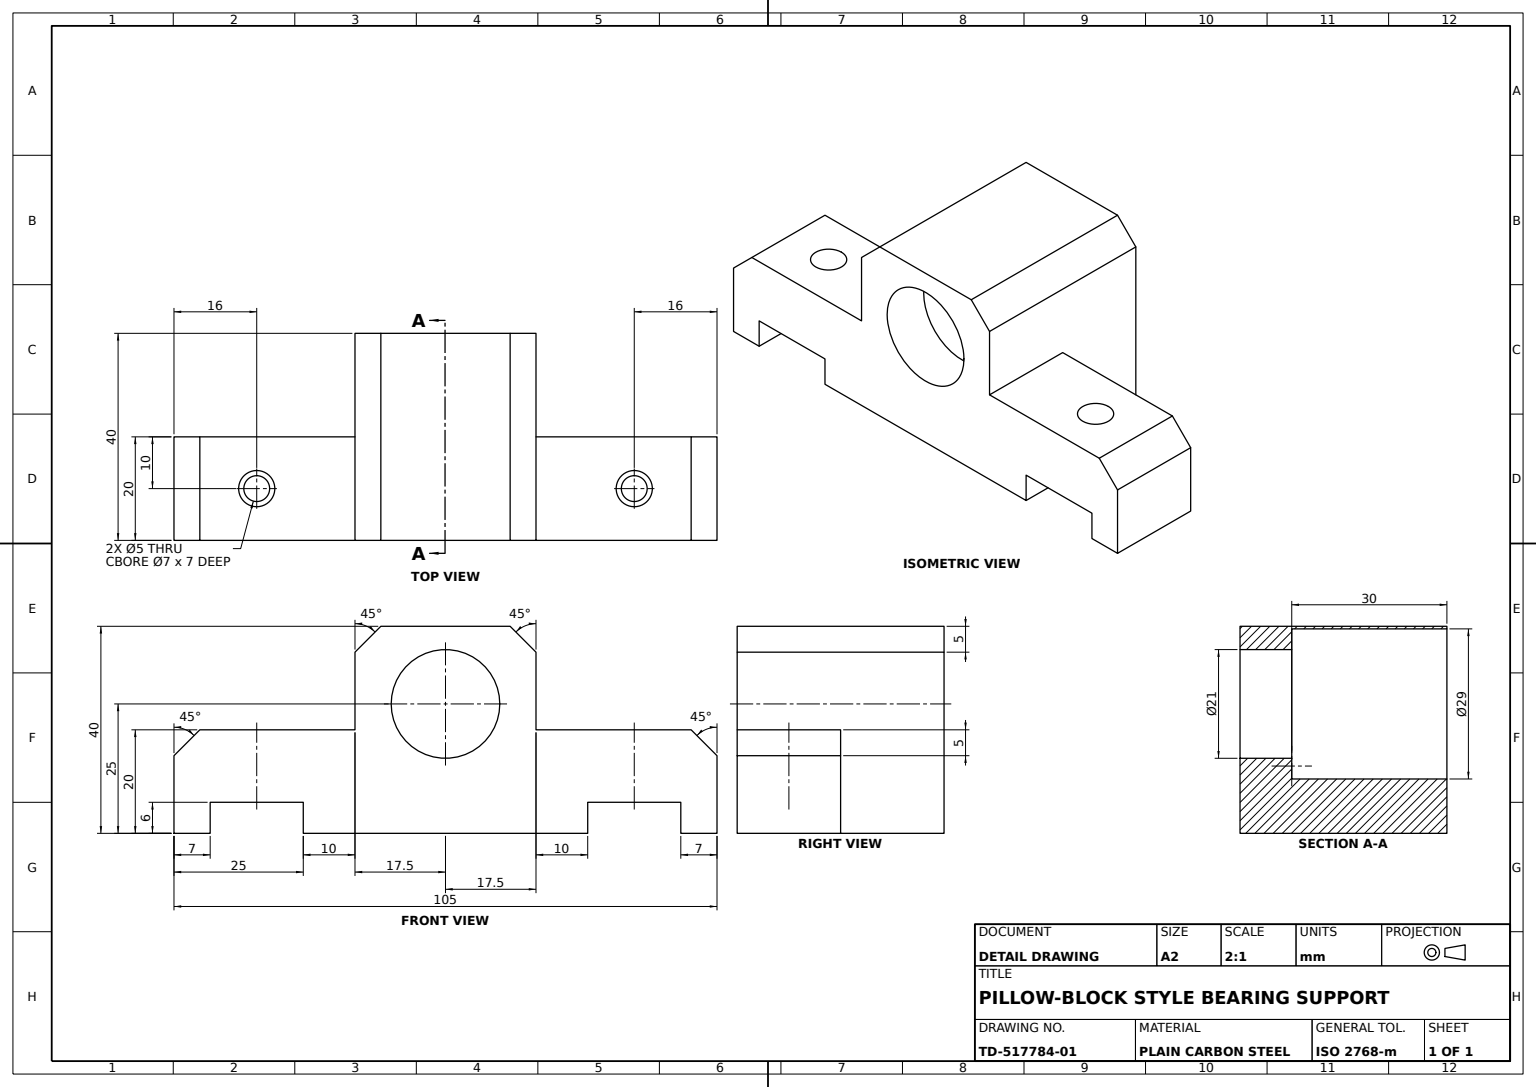
SolidWorks part; units mm, degrees
material "Plain Carbon Steel"
ref_plane "Front Plane" through (0, 0, 0) normal (0, 0, 1) x (1, 0, 0)
ref_plane "Top Plane" through (0, 0, 0) normal (0, 1, 0) x (1, 0, 0)
ref_plane "Right Plane" through (0, 0, 0) normal (1, 0, 0) x (0, 0, -1)
sketch "Base Body Profile" plane through (0, 0, 0) normal (0, 0, 1) x (1, 0, 0)
  line L0 (0, 0) -> (35, 0)
  line L1 (35, 0) -> (35, 35)
  line L2 (30, 40) -> (5, 40)
  line L3 (0, 35) -> (0, 0)
  line L6 (5, 40) -> (0, 35)
  line L10 (35, 35) -> (30, 40)
  dimension "D1" = 5
  dimension "D2" = 30
extrude "Base Body" add sketch "Base Body Profile" along normal blind 40
sketch "Mounting Lug 1 Profile" plane through (0, 0, 40) normal (0, 0, 1) x (1, 0, 0)
  line L0 (0, 0) -> (0, 20)
  line L1 (0, 35) -> (0, 0) construction
  line L2 (0, 20) -> (-19, 20)
  line L3 (-19, 20) -> (-28, 20)
  line L4 (-28, 20) -> (-30, 20)
  line L5 (-35, 15) -> (-35, 0)
  line L6 (-35, 0) -> (0, 0)
  line L8 (-35, 15) -> (-30, 20)
  line L9 (0, 0) -> (35, 0) construction
  dimension "D1" = 19
  dimension "D2" = 28
  dimension "D3" = 30
  dimension "D4" = 35
  dimension "D5" = 15
  dimension "D6" = 20
extrude "Mounting Lug 1" add sketch "Mounting Lug 1 Profile" against normal blind 20
sketch "Mounting Lug 2 Profile" plane through (0, 0, 40) normal (0, 0, 1) x (1, 0, 0)
  line L0 (35, 0) -> (35, 20)
  line L1 (35, 0) -> (35, 35) construction
  line L2 (35, 20) -> (54, 20)
  line L3 (54, 20) -> (63, 20)
  line L4 (63, 20) -> (65, 20)
  line L5 (70, 15) -> (70, 0)
  line L6 (70, 0) -> (35, 0)
  line L8 (70, 15) -> (65, 20)
  line L9 (-35, 15) -> (-35, 0) construction
  line L10 (-35, 0) -> (35, 0) construction
  dimension "D1" = 9
  dimension "D2" = 89
  dimension "D3" = 100
  dimension "D4" = 35
  dimension "D5" = 45
  dimension "D6" = 15
extrude "Mounting Lug 2" add sketch "Mounting Lug 2 Profile" against normal blind 20
sketch "Lug 2 Bottom Slot Profile" plane through (0, 0, 20) normal (0, 0, -1) x (-1, 0, 0)
  line L0 (-35, 20) -> (-35, 0) construction
  line L1 (-35, 0) -> (-70, 0) construction
  line L2 (-63, 0) -> (-63, 6)
  line L3 (-63, 6) -> (-45, 6)
  line L4 (-45, 6) -> (-45, 0)
  line L5 (-45, 0) -> (-63, 0)
  dimension "D1" = 10
  dimension "D2" = 28
  dimension "D3" = 6
extrude "Lug 2 Bottom Slot" cut sketch "Lug 2 Bottom Slot Profile" against normal blind 20
sketch "Lug 1 Bottom Slot Profile" plane through (0, 0, 20) normal (0, 0, -1) x (-1, 0, 0)
  line L0 (35, 0) -> (28, 0)
  line L1 (35, 0) -> (0, 0) construction
  line L2 (28, 0) -> (28, 6)
  line L3 (28, 6) -> (10, 6)
  line L4 (10, 6) -> (10, 0)
  line L5 (10, 0) -> (28, 0)
  line L6 (35, 15) -> (35, 0) construction
  line M1 (0, 0) -> (35, 0)
  dimension "D1" = 7
  dimension "D2" = 25
  dimension "D3" = 6
extrude "Lug 1 Bottom Slot" cut sketch "Lug 1 Bottom Slot Profile" against normal blind 20 contours L3 L4 L2 M1
sketch "Lug 2 Hole Ø7 Sketch" plane through (0, 20, 0) normal (0, 1, 0) x (1, 0, 0)
  line L0 (65, -40) -> (35, -40) construction
  line L1 (30, -40) -> (5, -40) construction
  circle A0 centre (54, -30) radius 3.5
  point P6 (17.5, -40)
  dimension "D1" = 7
  dimension "D4" = 7
  dimension "D2" = 10
  dimension "D3" = 36.5
extrude "Lug 2 Hole Ø7" cut sketch "Lug 2 Hole Ø7 Sketch" against normal blind 7
sketch "Lug 2 Hole Ø5 Sketch" plane through (0, 13, 0) normal (0, 1, 0) x (1, 0, 0)
  circle A0 centre (54, -30) radius 2.5
  dimension "D1" = 5
  dimension "D2" = 5
extrude "Lug 2 Hole Ø5" cut sketch "Lug 2 Hole Ø5 Sketch" against normal blind 7
sketch "Lug 1 Hole Ø7 Sketch" plane through (0, 20, 0) normal (0, 1, 0) x (1, 0, 0)
  line L0 (0, -40) -> (-30, -40) construction
  line L1 (30, 0) -> (5, 0) construction
  circle A0 centre (-19, -30) radius 3.5
  point P6 (17.5, 0)
  dimension "D1" = 7
  dimension "D4" = 7
  dimension "D2" = 10
  dimension "D3" = 36.5
extrude "Lug 1 Hole Ø7" cut sketch "Lug 1 Hole Ø7 Sketch" against normal blind 7
sketch "Lug 1 Hole Ø5 Sketch" plane through (0, 13, 0) normal (0, 1, 0) x (1, 0, 0)
  circle A0 centre (-19, -30) radius 2.5
  dimension "D1" = 5
  dimension "D2" = 5
extrude "Lug 1 Hole Ø5" cut sketch "Lug 1 Hole Ø5 Sketch" against normal blind 7
sketch "Bearing Bore Ø29 Sketch" plane through (0, 0, 0) normal (0, 0, -1) x (-1, 0, 0)
  line L0 (0, 35) -> (0, 0) construction
  line L1 (-30, 40) -> (-5, 40) construction
  circle A0 centre (-17.5, 25) radius 14.5
  dimension "D1" = 29
  dimension "D2" = 29
  dimension "D3" = 17.5
  dimension "D4" = 15
extrude "Bearing Bore Ø29" cut sketch "Bearing Bore Ø29 Sketch" against normal blind 30
sketch "Through Bore Ø21 Sketch" plane through (0, 0, 30) normal (0, 0, -1) x (-1, 0, 0)
  circle A0 centre (-17.5, 25) radius 10.5
  dimension "D1" = 21
  dimension "D2" = 21
extrude "Through Bore Ø21" cut sketch "Through Bore Ø21 Sketch" against normal through all
